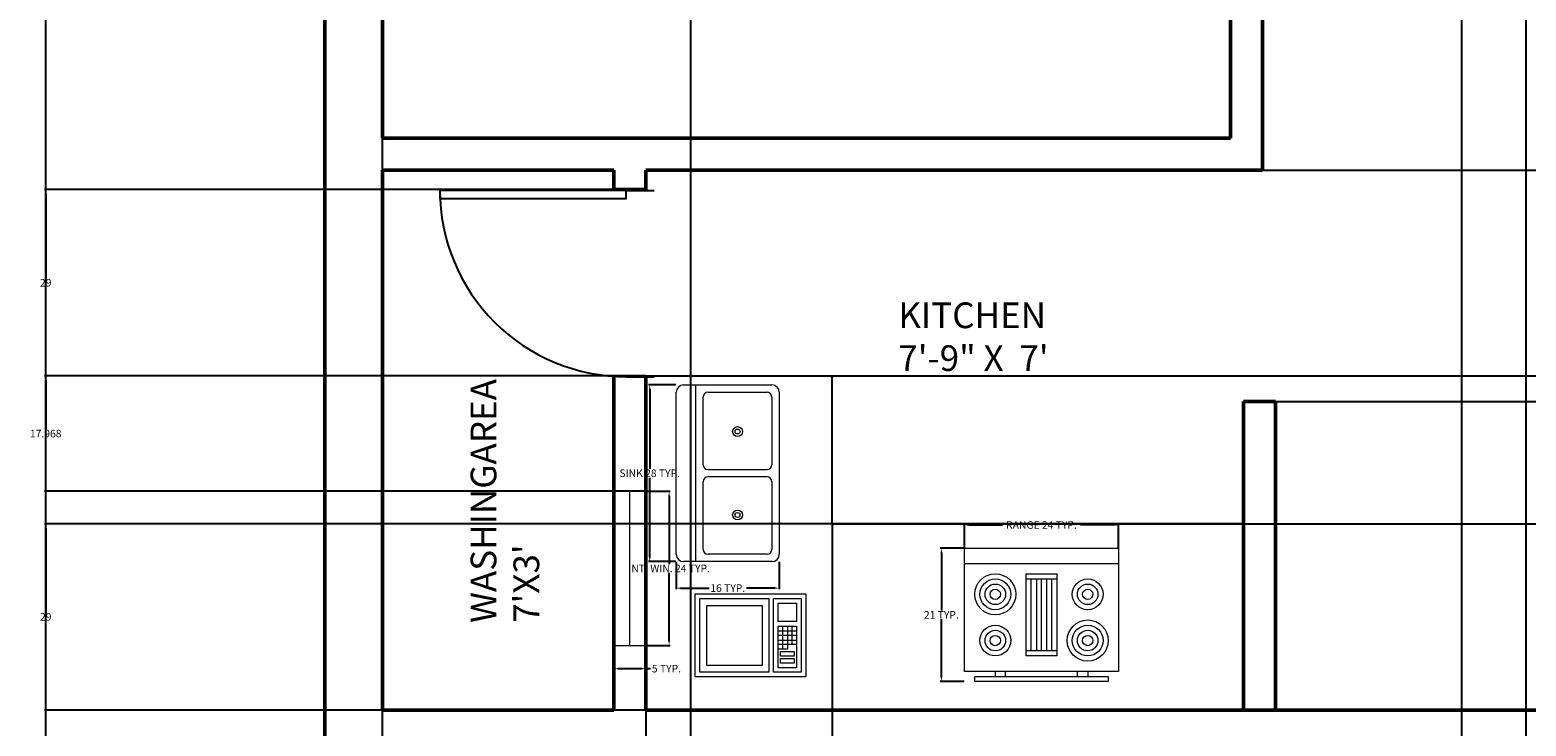
# Model space of a CAD drawing. Units: inches. Extents: x 3506 to 3958, y 1553 to 2506.
# Tile 13 of 16: x 3506 to 3739, y 2229 to 2337. Entities that reach past the tile are written whole.
import ezdxf

# ---------------------------------------------------------------- set-up
doc = ezdxf.new("R2010")
doc.units = ezdxf.units.IN
doc.header["$MEASUREMENT"] = 0
for name, color, linetype, lineweight in [('A-ANNO-DIMS', 2, 'Continuous', 18), ('A-AREA-IDEN', 7, 'Continuous', 18), ('A-FLOR-CASE', 7, 'Continuous', 25), ('A-WALL', 7, 'Continuous', 50), ('doors', 40, 'Continuous', 25), ('kitchen', 181, 'Continuous', 18), ('window', 30, 'Continuous', 20)]:
    doc.layers.add(name, color=color, linetype=linetype, lineweight=lineweight)
doc.layers.add('A-WALL-PATT', color=251, linetype='Continuous', lineweight=13, true_color=0x636466)
doc.styles.get("Standard").update_dxf_attribs({"font": 'arial.ttf'})
doc.dimstyles.get("Standard").update_dxf_attribs({"dimtxt": 1.18, "dimasz": 0.68, "dimexe": 0.18, "dimexo": 0.0625, "dimgap": 0.09, "dimtad": 0, "dimtih": 1, "dimtoh": 1, "dimdec": 1, "dimzin": 0, "dimdsep": 46, "dimlunit": 3, "dimtxsty": 'Standard', "dimcen": 0.09, "dimadec": 0, "dimazin": 0, "dimtfac": 1, "dimtdec": 1, "dimtofl": 0, "dimtmove": 0, "dimatfit": 3, "dimfxl": 1, "dimtolj": 1, "dimtzin": 0, "dimarcsym": 0})

# ---------------------------------------------------------------- blocks, each defined once
blk = doc.blocks.new('*U12')
for p, q in [((0, 0), (0, 6)), ((40, 0), (40, 6))]:
    blk.add_line(p, q)
blk.add_lwpolyline([(0, 0), (0, -40), (1.75, -40), (1.75, 0)], close=True)
blk.add_arc((0, 0), 40, 270, 0)
blk = doc.blocks.new('Microwave')
for p, q in [((18, 10), (22, 10)), ((19, 7), (19, 11)), ((20, 11), (20, 7)), ((21, 7), (21, 11)), ((22, 9), (18, 9)), ((18, 8), (22, 8)), ((22, 7), (18, 7)), ((19, 6), (19, 7)), ((20, 7), (20, 6)), ((20, 6), (18, 6))]:
    blk.add_line(p, q)
for points in [[(0, 0), (0, 18), (24, 18), (24, 0)], [(1, 1), (1, 17), (16, 17), (16, 1)], [(17, 1), (17, 17), (23, 17), (23, 1)], [(2.5, 2.5), (2.5, 15.5), (14.5, 15.5), (14.5, 2.5)], [(18, 12), (18, 16), (22, 16), (22, 12)], [(18, 2), (18, 11), (22, 11), (22, 2)], [(18.5, 4.5), (18.5, 5.5), (21.5, 5.5), (21.5, 4.5)], [(18.5, 3), (18.5, 4), (21.5, 4), (21.5, 3)]]:
    blk.add_lwpolyline(points, close=True)
blk = doc.blocks.new('Range-Oven - 30 in top')
for p, q in [((0, -3), (30, -3)), ((12, -6), (18, -6)), ((13, -20), (13, -6)), ((14, -6), (14, -20)), ((15, -20), (15, -6)), ((16, -6), (16, -20)), ((17, -20), (17, -6)), ((18, -20), (12, -20)), ((6, -24), (6, -25)), ((8, -25), (8, -24)), ((22, -25), (22, -24)), ((24, -24), (24, -25))]:
    blk.add_line(p, q)
for points in [[(0, -24), (0, 0), (30, 0), (30, -24)], [(12, -21), (12, -5), (18, -5), (18, -21)], [(2, -26), (2, -25), (28, -25), (28, -26)]]:
    blk.add_lwpolyline(points, close=True)
for centre, radius in [((6, -9), 4), ((6, -9), 3), ((6, -9), 2), ((6, -9), 1), ((24, -9), 3), ((24, -9), 2), ((24, -9), 1), ((24, -18), 4), ((6, -18), 3), ((6, -18), 2), ((6, -18), 1), ((24, -18), 3), ((24, -18), 2), ((24, -18), 1)]:
    blk.add_circle(centre, radius)
blk = doc.blocks.new('Sink-double - 36 in top')
for p, q in [((-18, -4), (18, -4)), ((-0.75, -18.5), (-0.75, -6.5)), ((0.75, -6.5), (0.75, -18.5))]:
    blk.add_line(p, q)
for points in [[(-16.5, 0), (16.5, 0)], [(-18, -19.5), (-18, -1.5)], [(18, -1.5), (18, -19.5)], [(-15.5, -5.5), (-1.75, -5.5)], [(1.75, -5.5), (15.5, -5.5)], [(-16.5, -18.5), (-16.5, -6.5)], [(16.5, -6.5), (16.5, -18.5)], [(16.5, -21), (-16.5, -21)], [(-1.75, -19.5), (-15.5, -19.5)], [(15.5, -19.5), (1.75, -19.5)]]:
    blk.add_lwpolyline(points)
for centre, radius in [((-8.5, -12.5), 1), ((-8.5, -12.5), 0.5), ((8.5, -12.5), 1), ((8.5, -12.5), 0.5)]:
    blk.add_circle(centre, radius)
for centre, radius, start, end in [((-16.5, -1.5), 1.5, 90, 180), ((16.5, -1.5), 1.5, 0, 90), ((-15.5, -6.5), 1, 90, 180), ((-1.75, -6.5), 1, 0, 90), ((1.75, -6.5), 1, 90, 180), ((15.5, -6.5), 1, 0, 90), ((-16.5, -19.5), 1.5, 180, 270), ((-15.5, -18.5), 1, 180, 270), ((-1.75, -18.5), 1, 270, 0), ((1.75, -18.5), 1, 180, 270), ((15.5, -18.5), 1, 270, 0), ((16.5, -19.5), 1.5, 270, 0)]:
    blk.add_arc(centre, radius, start, end)
blk = doc.blocks.new('WIN-24IN-5IN-PARTITION')
for p, q in [((5, 24), (0, 24)), ((0, 24), (0, 0)), ((2.5, 0), (2.5, 24)), ((5, 0), (5, 24)), ((0, 0), (5, 0)), ((0, 0), (2.5, 0))]:
    blk.add_line(p, q)
blk = doc.blocks.new('*D22')
at = {"layer": 'A-ANNO-DIMS', "color": 0, "lineweight": -2, "transparency": 16777216}
for p, q in [((3651.31, 2256.65), (3651.31, 2260.37)), ((3651.99, 2260.19), (3657.21, 2260.19)), ((3674.61, 2260.19), (3669.39, 2260.19)), ((3675.29, 2256.65), (3675.29, 2260.37))]:
    blk.add_line(p, q, dxfattribs=at)
at = {"layer": 'A-ANNO-DIMS', "color": 0, "transparency": 16777216}
for points in [[(3651.99, 2260.3), (3651.99, 2260.07), (3651.31, 2260.19)], [(3674.61, 2260.3), (3674.61, 2260.07), (3675.29, 2260.19)]]:
    blk.add_solid(points, dxfattribs=at)
at = {"layer": 'Defpoints', "color": 0, "transparency": 16777216}
for p in [(3675.29, 2260.19), (3651.31, 2256.59), (3675.29, 2256.59)]:
    blk.add_point(p, dxfattribs=at)
at = {"layer": 'A-ANNO-DIMS', "color": 0, "transparency": 16777216, "insert": (3663.3, 2260.19), "char_height": 1.18, "attachment_point": 5}
blk.add_mtext('\\A1;RANGE 24 TYP.', dxfattribs=at)
blk = doc.blocks.new('*D23')
at = {"layer": 'A-ANNO-DIMS', "color": 0, "lineweight": -2, "transparency": 16777216}
for p, q in [((3651.25, 2256.59), (3647.53, 2256.59)), ((3647.71, 2255.91), (3647.71, 2246.88)), ((3647.71, 2236.49), (3647.71, 2245.52)), ((3651.25, 2235.81), (3647.53, 2235.81))]:
    blk.add_line(p, q, dxfattribs=at)
at = {"layer": 'A-ANNO-DIMS', "color": 0, "transparency": 16777216}
for points in [[(3647.6, 2255.91), (3647.83, 2255.91), (3647.71, 2256.59)], [(3647.6, 2236.49), (3647.83, 2236.49), (3647.71, 2235.81)]]:
    blk.add_solid(points, dxfattribs=at)
at = {"layer": 'Defpoints', "color": 0, "transparency": 16777216}
for p in [(3647.71, 2256.59), (3651.31, 2256.59), (3651.31, 2235.81)]:
    blk.add_point(p, dxfattribs=at)
at = {"layer": 'A-ANNO-DIMS', "color": 0, "transparency": 16777216, "insert": (3647.71, 2246.2), "char_height": 1.18, "attachment_point": 5}
blk.add_mtext('\\A1;21 TYP.', dxfattribs=at)
blk = doc.blocks.new('*D24')
at = {"layer": 'A-ANNO-DIMS', "color": 0, "lineweight": -2, "transparency": 16777216}
for p, q in [((3606.38, 2281.99), (3602.13, 2281.99)), ((3602.31, 2281.31), (3602.31, 2268.94)), ((3602.31, 2255.17), (3602.31, 2267.54)), ((3606.38, 2254.49), (3602.13, 2254.49))]:
    blk.add_line(p, q, dxfattribs=at)
at = {"layer": 'A-ANNO-DIMS', "color": 0, "transparency": 16777216}
for points in [[(3602.2, 2281.31), (3602.43, 2281.31), (3602.31, 2281.99)], [(3602.2, 2255.17), (3602.43, 2255.17), (3602.31, 2254.49)]]:
    blk.add_solid(points, dxfattribs=at)
at = {"layer": 'Defpoints', "color": 0, "transparency": 16777216}
for p in [(3602.31, 2281.99), (3606.44, 2281.99), (3606.44, 2254.49)]:
    blk.add_point(p, dxfattribs=at)
at = {"layer": 'A-ANNO-DIMS', "color": 0, "transparency": 16777216, "insert": (3602.31, 2268.24), "char_height": 1.18, "attachment_point": 5}
blk.add_mtext('\\A1;SINK 28 TYP.', dxfattribs=at)
blk = doc.blocks.new('*D25')
at = {"layer": 'A-ANNO-DIMS', "color": 0, "lineweight": -2, "transparency": 16777216}
for p, q in [((3606.44, 2254.43), (3606.44, 2250.18)), ((3622.48, 2254.43), (3622.48, 2250.18)), ((3607.12, 2250.36), (3611.55, 2250.36)), ((3621.8, 2250.36), (3617.36, 2250.36))]:
    blk.add_line(p, q, dxfattribs=at)
at = {"layer": 'A-ANNO-DIMS', "color": 0, "transparency": 16777216}
for points in [[(3607.12, 2250.48), (3607.12, 2250.25), (3606.44, 2250.36)], [(3621.8, 2250.48), (3621.8, 2250.25), (3622.48, 2250.36)]]:
    blk.add_solid(points, dxfattribs=at)
at = {"layer": 'Defpoints', "color": 0, "transparency": 16777216}
for p in [(3606.44, 2254.49), (3622.48, 2254.49), (3606.44, 2250.36)]:
    blk.add_point(p, dxfattribs=at)
at = {"layer": 'A-ANNO-DIMS', "color": 0, "transparency": 16777216, "insert": (3614.46, 2250.36), "char_height": 1.18, "attachment_point": 5}
blk.add_mtext('\\A1;16 TYP.', dxfattribs=at)
blk = doc.blocks.new('*D34')
at = {"layer": 'A-ANNO-DIMS', "color": 0, "lineweight": -2, "transparency": 16777216}
for p, q in [((3601.79, 2265.43), (3605.51, 2265.43)), ((3605.33, 2264.75), (3605.33, 2254.11)), ((3605.33, 2242.11), (3605.33, 2252.74)), ((3601.79, 2241.43), (3605.51, 2241.43))]:
    blk.add_line(p, q, dxfattribs=at)
at = {"layer": 'A-ANNO-DIMS', "color": 0, "transparency": 16777216}
for points in [[(3605.22, 2264.75), (3605.44, 2264.75), (3605.33, 2265.43)], [(3605.22, 2242.11), (3605.44, 2242.11), (3605.33, 2241.43)]]:
    blk.add_solid(points, dxfattribs=at)
at = {"layer": 'Defpoints', "color": 0, "transparency": 16777216}
for p in [(3601.73, 2265.43), (3605.33, 2265.43), (3601.73, 2241.43)]:
    blk.add_point(p, dxfattribs=at)
at = {"layer": 'A-ANNO-DIMS', "color": 0, "transparency": 16777216, "insert": (3605.33, 2253.43), "char_height": 1.18, "attachment_point": 5}
blk.add_mtext('\\A1;INT. WIN. 24 TYP.', dxfattribs=at)
blk = doc.blocks.new('*D35')
at = {"layer": 'A-ANNO-DIMS', "color": 0, "lineweight": -2, "transparency": 16777216}
for p, q in [((3596.73, 2241.36), (3596.73, 2237.65)), ((3601.73, 2241.36), (3601.73, 2237.65)), ((3597.41, 2237.83), (3601.05, 2237.83)), ((3601.73, 2237.83), (3602.41, 2237.83))]:
    blk.add_line(p, q, dxfattribs=at)
at = {"layer": 'A-ANNO-DIMS', "color": 0, "transparency": 16777216}
for points in [[(3597.41, 2237.94), (3597.41, 2237.71), (3596.73, 2237.83)], [(3601.05, 2237.94), (3601.05, 2237.71), (3601.73, 2237.83)]]:
    blk.add_solid(points, dxfattribs=at)
at = {"layer": 'Defpoints', "color": 0, "transparency": 16777216}
for p in [(3596.73, 2241.43), (3601.73, 2241.43), (3601.73, 2237.83)]:
    blk.add_point(p, dxfattribs=at)
at = {"layer": 'A-ANNO-DIMS', "color": 0, "transparency": 16777216, "insert": (3604.91, 2237.83), "char_height": 1.18, "attachment_point": 5}
blk.add_mtext('\\A1;5 TYP.', dxfattribs=at)
blk = doc.blocks.new('*D44')
at = {"layer": 'A-ANNO-DIMS', "color": 0, "lineweight": -2, "transparency": 16777216}
for p, q in [((3911.67, 2461.39), (3508.1, 2461.39)), ((3508.28, 2460.71), (3508.28, 2344.59)), ((3508.28, 2227.07), (3508.28, 2343.2)), ((3560.67, 2226.39), (3508.1, 2226.39))]:
    blk.add_line(p, q, dxfattribs=at)
at = {"layer": 'A-ANNO-DIMS', "color": 0, "transparency": 16777216}
for points in [[(3508.17, 2460.71), (3508.39, 2460.71), (3508.28, 2461.39)], [(3508.17, 2227.07), (3508.39, 2227.07), (3508.28, 2226.39)]]:
    blk.add_solid(points, dxfattribs=at)
at = {"layer": 'Defpoints', "color": 0, "transparency": 16777216}
for p in [(3508.28, 2461.39), (3911.73, 2461.39), (3560.73, 2226.39)]:
    blk.add_point(p, dxfattribs=at)
at = {"layer": 'A-ANNO-DIMS', "color": 0, "transparency": 16777216, "insert": (3508.28, 2343.89), "char_height": 1.18, "attachment_point": 5}
blk.add_mtext('\\A1;235', dxfattribs=at)
blk = doc.blocks.new('*D50')
at = {"layer": 'A-ANNO-DIMS', "color": 0, "lineweight": -2, "transparency": 16777216}
for p, q in [((3608.73, 1606.46), (3608.73, 2505.02)), ((3609.41, 2504.84), (3672.39, 2504.84)), ((3738.05, 2504.84), (3675.07, 2504.84)), ((3738.73, 1606.46), (3738.73, 2505.02))]:
    blk.add_line(p, q, dxfattribs=at)
at = {"layer": 'A-ANNO-DIMS', "color": 0, "transparency": 16777216}
for points in [[(3609.41, 2504.96), (3609.41, 2504.73), (3608.73, 2504.84)], [(3738.05, 2504.96), (3738.05, 2504.73), (3738.73, 2504.84)]]:
    blk.add_solid(points, dxfattribs=at)
at = {"layer": 'Defpoints', "color": 0, "transparency": 16777216}
for p in [(3738.73, 2504.84), (3608.73, 1606.39), (3738.73, 1606.39)]:
    blk.add_point(p, dxfattribs=at)
at = {"layer": 'A-ANNO-DIMS', "color": 0, "transparency": 16777216, "insert": (3673.73, 2504.84), "char_height": 1.18, "attachment_point": 5}
blk.add_mtext('\\A1;130', dxfattribs=at)
blk = doc.blocks.new('*D52')
at = {"layer": 'A-ANNO-DIMS', "color": 0, "lineweight": -2, "transparency": 16777216}
for p, q in [((3560.73, 1606.46), (3560.73, 2505.02)), ((3561.41, 2504.84), (3583.77, 2504.84)), ((3608.05, 2504.84), (3585.69, 2504.84)), ((3608.73, 1606.46), (3608.73, 2505.02))]:
    blk.add_line(p, q, dxfattribs=at)
at = {"layer": 'A-ANNO-DIMS', "color": 0, "transparency": 16777216}
for points in [[(3561.41, 2504.96), (3561.41, 2504.73), (3560.73, 2504.84)], [(3608.05, 2504.96), (3608.05, 2504.73), (3608.73, 2504.84)]]:
    blk.add_solid(points, dxfattribs=at)
at = {"layer": 'Defpoints', "color": 0, "transparency": 16777216}
for p in [(3608.73, 2504.84), (3560.73, 1606.39), (3608.73, 1606.39)]:
    blk.add_point(p, dxfattribs=at)
at = {"layer": 'A-ANNO-DIMS', "color": 0, "transparency": 16777216, "insert": (3584.73, 2504.84), "char_height": 1.18, "attachment_point": 5}
blk.add_mtext('\\A1;48', dxfattribs=at)
blk = doc.blocks.new('*D58')
at = {"layer": 'A-ANNO-DIMS', "color": 0, "lineweight": -2, "transparency": 16777216}
for p, q in [((3596.67, 2312.39), (3508.1, 2312.39)), ((3508.28, 2311.71), (3508.28, 2298.59)), ((3508.28, 2284.07), (3508.28, 2297.2)), ((3596.67, 2283.39), (3508.1, 2283.39))]:
    blk.add_line(p, q, dxfattribs=at)
at = {"layer": 'A-ANNO-DIMS', "color": 0, "transparency": 16777216}
for points in [[(3508.17, 2311.71), (3508.39, 2311.71), (3508.28, 2312.39)], [(3508.17, 2284.07), (3508.39, 2284.07), (3508.28, 2283.39)]]:
    blk.add_solid(points, dxfattribs=at)
at = {"layer": 'Defpoints', "color": 0, "transparency": 16777216}
for p in [(3596.73, 2312.39), (3508.28, 2283.39), (3596.73, 2283.39)]:
    blk.add_point(p, dxfattribs=at)
at = {"layer": 'A-ANNO-DIMS', "color": 0, "transparency": 16777216, "insert": (3508.28, 2297.89), "char_height": 1.18, "attachment_point": 5}
blk.add_mtext('\\A1;29', dxfattribs=at)
blk = doc.blocks.new('*D59')
at = {"layer": 'A-ANNO-DIMS', "color": 0, "lineweight": -2, "transparency": 16777216}
for p, q in [((3728.73, 1689.46), (3728.73, 2505.02)), ((3729.41, 2504.84), (3732.85, 2504.84)), ((3738.05, 2504.84), (3734.61, 2504.84)), ((3738.73, 1689.46), (3738.73, 2505.02))]:
    blk.add_line(p, q, dxfattribs=at)
at = {"layer": 'A-ANNO-DIMS', "color": 0, "transparency": 16777216}
for points in [[(3729.41, 2504.96), (3729.41, 2504.73), (3728.73, 2504.84)], [(3738.05, 2504.96), (3738.05, 2504.73), (3738.73, 2504.84)]]:
    blk.add_solid(points, dxfattribs=at)
at = {"layer": 'Defpoints', "color": 0, "transparency": 16777216}
for p in [(3738.73, 2504.84), (3728.73, 1689.39), (3738.73, 1689.39)]:
    blk.add_point(p, dxfattribs=at)
at = {"layer": 'A-ANNO-DIMS', "color": 0, "transparency": 16777216, "insert": (3733.73, 2504.84), "char_height": 1.18, "attachment_point": 5}
blk.add_mtext('\\A1;10', dxfattribs=at)
blk = doc.blocks.new('*D67')
at = {"layer": 'A-ANNO-DIMS', "color": 0, "lineweight": -2, "transparency": 16777216}
for p, q in [((3697.79, 2315.39), (3955.36, 2315.39)), ((3955.18, 2314.71), (3955.18, 2298.09)), ((3955.18, 2280.07), (3955.18, 2296.7)), ((3699.79, 2279.39), (3955.36, 2279.39))]:
    blk.add_line(p, q, dxfattribs=at)
at = {"layer": 'A-ANNO-DIMS', "color": 0, "transparency": 16777216}
for points in [[(3955.07, 2314.71), (3955.29, 2314.71), (3955.18, 2315.39)], [(3955.07, 2280.07), (3955.29, 2280.07), (3955.18, 2279.39)]]:
    blk.add_solid(points, dxfattribs=at)
at = {"layer": 'Defpoints', "color": 0, "transparency": 16777216}
for p in [(3697.73, 2315.39), (3699.73, 2279.39), (3955.18, 2279.39)]:
    blk.add_point(p, dxfattribs=at)
at = {"layer": 'A-ANNO-DIMS', "color": 0, "transparency": 16777216, "insert": (3955.18, 2297.39), "char_height": 1.18, "attachment_point": 5}
blk.add_mtext('\\A1;36', dxfattribs=at)
blk = doc.blocks.new('*D68')
at = {"layer": 'A-ANNO-DIMS', "color": 0, "lineweight": -2, "transparency": 16777216}
for p, q in [((3630.73, 2260.33), (3630.73, 1553.76)), ((3601.73, 2231.33), (3601.73, 1553.76)), ((3602.41, 1553.94), (3615.28, 1553.94)), ((3630.05, 1553.94), (3617.18, 1553.94))]:
    blk.add_line(p, q, dxfattribs=at)
at = {"layer": 'A-ANNO-DIMS', "color": 0, "transparency": 16777216}
for points in [[(3602.41, 1554.06), (3602.41, 1553.83), (3601.73, 1553.94)], [(3630.05, 1554.06), (3630.05, 1553.83), (3630.73, 1553.94)]]:
    blk.add_solid(points, dxfattribs=at)
at = {"layer": 'Defpoints', "color": 0, "transparency": 16777216}
for p in [(3630.73, 2260.39), (3601.73, 2231.39), (3630.73, 1553.94)]:
    blk.add_point(p, dxfattribs=at)
at = {"layer": 'A-ANNO-DIMS', "color": 0, "transparency": 16777216, "insert": (3616.23, 1553.94), "char_height": 1.18, "attachment_point": 5}
blk.add_mtext('\\A1;29', dxfattribs=at)
blk = doc.blocks.new('*D69')
at = {"layer": 'A-ANNO-DIMS', "color": 0, "lineweight": -2, "transparency": 16777216}
for p, q in [((3630.79, 2283.39), (3955.36, 2283.39)), ((3955.18, 2282.71), (3955.18, 2272.59)), ((3955.18, 2261.07), (3955.18, 2271.2)), ((3630.79, 2260.39), (3955.36, 2260.39))]:
    blk.add_line(p, q, dxfattribs=at)
at = {"layer": 'A-ANNO-DIMS', "color": 0, "transparency": 16777216}
for points in [[(3955.07, 2282.71), (3955.29, 2282.71), (3955.18, 2283.39)], [(3955.07, 2261.07), (3955.29, 2261.07), (3955.18, 2260.39)]]:
    blk.add_solid(points, dxfattribs=at)
at = {"layer": 'Defpoints', "color": 0, "transparency": 16777216}
for p in [(3630.73, 2283.39), (3630.73, 2260.39), (3955.18, 2260.39)]:
    blk.add_point(p, dxfattribs=at)
at = {"layer": 'A-ANNO-DIMS', "color": 0, "transparency": 16777216, "insert": (3955.18, 2271.89), "char_height": 1.18, "attachment_point": 5}
blk.add_mtext('\\A1;23', dxfattribs=at)
blk = doc.blocks.new('*D70')
at = {"layer": 'A-ANNO-DIMS', "color": 0, "lineweight": -2, "transparency": 16777216}
for p, q in [((3694.67, 2260.39), (3508.1, 2260.39)), ((3508.28, 2259.71), (3508.28, 2246.59)), ((3508.28, 2232.07), (3508.28, 2245.2)), ((3694.67, 2231.39), (3508.1, 2231.39))]:
    blk.add_line(p, q, dxfattribs=at)
at = {"layer": 'A-ANNO-DIMS', "color": 0, "transparency": 16777216}
for points in [[(3508.17, 2259.71), (3508.39, 2259.71), (3508.28, 2260.39)], [(3508.17, 2232.07), (3508.39, 2232.07), (3508.28, 2231.39)]]:
    blk.add_solid(points, dxfattribs=at)
at = {"layer": 'Defpoints', "color": 0, "transparency": 16777216}
for p in [(3694.73, 2260.39), (3508.28, 2231.39), (3694.73, 2231.39)]:
    blk.add_point(p, dxfattribs=at)
at = {"layer": 'A-ANNO-DIMS', "color": 0, "transparency": 16777216, "insert": (3508.28, 2245.89), "char_height": 1.18, "attachment_point": 5}
blk.add_mtext('\\A1;29', dxfattribs=at)
blk = doc.blocks.new('*D71')
at = {"layer": 'A-ANNO-DIMS', "color": 0, "lineweight": -2, "transparency": 16777216}
for p, q in [((3601.67, 2283.39), (3508.1, 2283.39)), ((3508.28, 2282.71), (3508.28, 2275.1)), ((3508.28, 2266.11), (3508.28, 2273.72)), ((3601.67, 2265.43), (3508.1, 2265.43))]:
    blk.add_line(p, q, dxfattribs=at)
at = {"layer": 'A-ANNO-DIMS', "color": 0, "transparency": 16777216}
for points in [[(3508.17, 2282.71), (3508.39, 2282.71), (3508.28, 2283.39)], [(3508.17, 2266.11), (3508.39, 2266.11), (3508.28, 2265.43)]]:
    blk.add_solid(points, dxfattribs=at)
at = {"layer": 'Defpoints', "color": 0, "transparency": 16777216}
for p in [(3508.28, 2283.39), (3601.73, 2283.39), (3601.73, 2265.43)]:
    blk.add_point(p, dxfattribs=at)
at = {"layer": 'A-ANNO-DIMS', "color": 0, "transparency": 16777216, "insert": (3508.28, 2274.41), "char_height": 1.18, "attachment_point": 5}
blk.add_mtext('\\A1;17.968', dxfattribs=at)

msp = doc.modelspace()

# ---------------------------------------------------------------- hatches: boundary and pattern name
at = {"layer": 'A-WALL-PATT'}
h = msp.add_hatch(dxfattribs=at)
h.set_pattern_fill('ANSI31', color=256)
h.paths.add_polyline_path([(3911.7302, 2461.3942), (3551.7302, 2461.3942), (3551.7302, 2152.516), (3560.7302, 2152.516), (3560.7302, 2116.516), (3551.7302, 2116.516), (3551.7302, 1920.5711), (3556.2302, 1920.5711), (3560.7302, 1920.5711), (3560.7302, 2000.3942), (3692.7302, 2000.3942), (3692.7302, 1997.3942), (3697.7302, 1997.3942), (3697.7302, 2000.3942), (3771.7302, 2000.3942), (3771.7302, 1997.3942), (3776.7302, 1997.3942), (3776.7302, 1997.7206), (3778.5802, 1997.7206), (3807.5802, 1997.7206), (3807.5802, 1996.4519), (3778.5802, 1996.4519), (3778.5802, 1997.7206), (3776.7302, 1997.7206), (3776.7302, 1997.3942), (3771.7302, 1997.3942), (3771.7302, 2000.3942), (3697.7302, 2000.3942), (3697.7302, 1997.3942), (3692.7302, 1997.3942), (3689.8302, 1997.3942), (3689.8302, 1995.8192), (3653.8302, 1995.8192), (3653.8302, 1997.3942), (3689.8302, 1997.3942), (3692.7302, 1997.3942), (3692.7302, 2000.3942), (3560.7302, 2000.3942), (3560.7302, 1920.5711), (3551.7302, 1920.5711), (3551.7302, 1884.5711), (3551.7302, 1597.3942), (3911.7302, 1597.3942)], flags=17)
h.paths.add_polyline_path([(3596.7302, 2005.3942), (3596.7302, 2057.3035, -0.38730371), (3569.1778, 2085), (3569.15, 2085), (3569.15, 2086.2688), (3598.15, 2086.2688), (3598.15, 2085), (3569.1778, 2085, 0.38730371), (3596.7302, 2057.3035), (3596.7302, 2057.3942), (3601.7302, 2057.3942), (3601.7302, 2055.3942), (3630.7302, 2055.3942), (3630.7302, 2034.3942), (3694.7302, 2034.3942), (3694.7302, 2053.3942), (3699.7302, 2053.3942), (3699.7302, 2005.3942), (3860.7302, 2005.3942), (3860.7302, 2173.3942), (3771.7302, 2173.3942), (3771.7302, 2194.3942), (3776.7302, 2194.3942), (3776.7302, 2178.3942), (3860.7302, 2178.3942), (3860.7302, 2231.3942), (3601.7302, 2231.3942), (3601.7302, 2241.426), (3596.7302, 2241.426), (3596.7302, 2231.3942), (3560.7302, 2231.3942), (3560.7302, 2315.3942), (3596.7302, 2315.3942), (3596.7302, 2312.3942), (3601.7302, 2312.3942), (3601.7302, 2315.3942), (3697.7302, 2315.3942), (3697.7302, 2413.3942), (3692.7302, 2413.3942), (3692.7302, 2320.3942), (3560.7302, 2320.3942), (3560.7302, 2452.3942), (3692.7302, 2452.3942), (3692.7302, 2449.3942), (3697.7302, 2449.3942), (3697.7302, 2452.3942), (3771.7302, 2452.3942), (3771.7302, 2449.3942), (3776.7302, 2449.3942), (3776.7302, 2452.3942), (3860.7302, 2452.3942), (3860.7302, 2437.2075), (3865.2302, 2437.2075), (3865.2302, 2413.2075), (3860.7302, 2413.2075), (3860.7302, 2367.6976), (3865.2302, 2367.6976), (3869.7302, 2367.6976), (3869.7302, 2319.6976), (3860.7302, 2319.6976), (3860.7302, 2211.6248), (3869.7302, 2211.6248), (3869.7302, 2187.6248), (3860.7302, 2187.6248), (3860.7302, 2138.4346), (3865.2302, 2138.4346), (3869.7302, 2138.4346), (3869.7302, 2090.4346), (3860.7302, 2090.4346), (3860.7302, 1985.8449), (3869.7302, 1985.8449), (3869.7302, 1961.8449), (3860.7302, 1961.8449), (3860.7302, 1897.0756), (3865.2302, 1897.0756), (3869.7302, 1897.0756), (3869.7302, 1849.0756), (3860.7302, 1849.0756), (3860.7302, 1847.8112), (3860.7302, 1779.3942), (3596.7302, 1779.3942), (3596.7302, 1831.3942), (3601.7302, 1831.3942), (3601.7302, 1828.3942), (3630.7302, 1828.3942), (3630.7302, 1808.3942), (3691.7302, 1808.3942), (3691.7302, 1815.3942), (3696.7302, 1815.3942), (3696.7302, 1779.3942), (3860.7302, 1779.3942), (3860.7302, 1947.3942), (3771.7302, 1947.3942), (3771.7302, 1968.3942), (3776.7302, 1968.3942), (3776.7302, 1952.3942), (3860.7302, 1952.3942), (3860.7302, 2005.3942)], flags=0)
h.paths.add_polyline_path([(3596.7302, 2038.8546), (3601.7302, 2038.8546), (3601.7302, 2014.8546), (3596.7302, 2014.8546)], flags=0)
h.paths.add_polyline_path([(3564.1688, 2107), (3564.1688, 2167), (3644.1688, 2167), (3644.1688, 2107)], flags=0)
h.paths.add_polyline_path([(3607.0972, 2052.0208), (3620.8472, 2052.0208, -0.41421356), (3621.9931, 2050.875), (3621.9931, 2025.6667, -0.41421356), (3620.8472, 2024.5208), (3607.0972, 2024.5208, -0.41421356), (3605.9514, 2025.6667), (3605.9514, 2050.875, -0.41421356)], flags=0)
h.paths.add_polyline_path([(3578.5688, 2115), (3565.3688, 2115), (3565.3688, 2135.8), (3578.5688, 2135.8), (3578.5688, 2138.2), (3565.3688, 2138.2), (3565.3688, 2159), (3580.5688, 2159), (3580.5688, 2153.8), (3593.7688, 2167), (3593.7688, 2151.8), (3578.5688, 2151.8)], flags=0)
h.paths.add_polyline_path([(3610.9167, 2050.875), (3620.0833, 2050.875, -0.41421356), (3620.8472, 2050.1111), (3620.8472, 2039.6076, -0.41421356), (3620.0833, 2038.8438), (3610.9167, 2038.8438, -0.41421356), (3610.1528, 2039.6076), (3610.1528, 2050.1111, -0.41421356)], flags=0)
h.paths.add_polyline_path([(3610.9167, 2037.6979), (3620.0833, 2037.6979, -0.41421356), (3620.8472, 2036.934), (3620.8472, 2026.4306, -0.41421356), (3620.0833, 2025.6667), (3610.9167, 2025.6667, -0.41421356), (3610.1528, 2026.4306), (3610.1528, 2036.934, -0.41421356)], flags=0)
h.paths.add_polyline_path([(3616.2639, 2044.7639, -1), (3614.7361, 2044.7639, -1)], flags=0)
h.paths.add_polyline_path([(3615.8819, 2044.7639, -1), (3615.1181, 2044.7639, -1)], flags=0)
h.paths.add_polyline_path([(3616.2639, 2031.7778, -1), (3614.7361, 2031.7778, -1)], flags=0)
h.paths.add_polyline_path([(3615.8819, 2031.7778, -1), (3615.1181, 2031.7778, -1)], flags=0)
h.paths.add_polyline_path([(3609.7539, 2021.7868), (3626.9586, 2021.7868), (3626.9586, 2008.8833), (3609.7539, 2008.8833)], flags=0)
h.paths.add_polyline_path([(3610.4708, 2021.07), (3621.2237, 2021.07), (3621.2237, 2009.6002), (3610.4708, 2009.6002)], flags=0)
h.paths.add_polyline_path([(3611.5461, 2019.9947), (3620.1484, 2019.9947), (3620.1484, 2010.6755), (3611.5461, 2010.6755)], flags=0)
h.paths.add_polyline_path([(3621.9405, 2021.07), (3626.2417, 2021.07), (3626.2417, 2009.6002), (3621.9405, 2009.6002)], flags=0)
h.paths.add_polyline_path([(3622.6574, 2020.3531), (3625.5248, 2020.3531), (3625.5248, 2017.4857), (3622.6574, 2017.4857)], flags=0)
h.paths.add_polyline_path([(3622.6574, 2016.7688), (3625.5248, 2016.7688), (3625.5248, 2010.317), (3622.6574, 2010.317)], flags=0)
h.paths.add_polyline_path([(3624.808, 2016.0519), (3624.808, 2013.9013), (3624.0911, 2013.9013), (3624.0911, 2013.1845), (3623.3743, 2013.1845), (3623.3743, 2013.9013), (3623.3743, 2016.0519)], flags=0)
h.paths.add_polyline_path([(3623.0158, 2012.8261), (3625.1664, 2012.8261), (3625.1664, 2012.1092), (3623.0158, 2012.1092)], flags=0)
h.paths.add_polyline_path([(3623.0158, 2011.7508), (3625.1664, 2011.7508), (3625.1664, 2011.0339), (3623.0158, 2011.0339)], flags=0)
h.paths.add_polyline_path([(3650.0591, 2031.8202), (3674.0368, 2031.8202), (3674.0368, 2012.638), (3669.2413, 2012.638), (3669.2413, 2011.8388), (3672.4383, 2011.8388), (3672.4383, 2011.0395), (3651.6576, 2011.0395), (3651.6576, 2011.8388), (3654.8546, 2011.8388), (3654.8546, 2012.638), (3650.0591, 2012.638)], flags=0)
h.paths.add_polyline_path([(3658.0517, 2024.6269, -1), (3651.6576, 2024.6269, -1)], flags=0)
h.paths.add_polyline_path([(3657.2524, 2024.6269, -1), (3652.4569, 2024.6269, -1)], flags=0)
h.paths.add_polyline_path([(3656.4532, 2024.6269, -1), (3653.2561, 2024.6269, -1)], flags=0)
h.paths.add_polyline_path([(3655.6539, 2024.6269, -1), (3654.0554, 2024.6269, -1)], flags=0)
h.paths.add_polyline_path([(3657.2524, 2017.4336, -1), (3652.4569, 2017.4336, -1)], flags=0)
h.paths.add_polyline_path([(3656.4532, 2017.4336, -1), (3653.2561, 2017.4336, -1)], flags=0)
h.paths.add_polyline_path([(3655.6539, 2017.4336, -1), (3654.0554, 2017.4336, -1)], flags=0)
h.paths.add_polyline_path([(3659.6502, 2027.8239), (3664.4457, 2027.8239), (3664.4457, 2015.0358), (3659.6502, 2015.0358)], flags=0)
h.paths.add_polyline_path([(3663.6465, 2027.0247), (3663.6465, 2015.8351), (3660.4494, 2015.8351), (3660.4494, 2027.0247)], flags=0)
h.paths.add_polyline_path([(3562.6688, 1945.5), (3642.6688, 1945.5), (3642.6688, 1885.5), (3562.6688, 1885.5)], flags=0)
h.paths.add_polyline_path([(3671.6391, 2024.6269, -1), (3666.8435, 2024.6269, -1)], flags=0)
h.paths.add_polyline_path([(3670.8398, 2024.6269, -1), (3667.6428, 2024.6269, -1)], flags=0)
h.paths.add_polyline_path([(3672.4383, 2017.4336, -1), (3666.0443, 2017.4336, -1)], flags=0)
h.paths.add_polyline_path([(3670.0405, 2024.6269, -1), (3668.442, 2024.6269, -1)], flags=0)
h.paths.add_polyline_path([(3671.6391, 2017.4336, -1), (3666.8435, 2017.4336, -1)], flags=0)
h.paths.add_polyline_path([(3670.8398, 2017.4336, -1), (3667.6428, 2017.4336, -1)], flags=0)
h.paths.add_polyline_path([(3592.2688, 1945.5), (3592.2688, 1930.3), (3577.0688, 1930.3), (3577.0688, 1893.5), (3563.8688, 1893.5), (3563.8688, 1914.3), (3577.0688, 1914.3), (3577.0688, 1916.7), (3563.8688, 1916.7), (3563.8688, 1937.5), (3579.0688, 1937.5), (3579.0688, 1932.3)], flags=0)
h.paths.add_polyline_path([(3670.0405, 2017.4336, -1), (3668.442, 2017.4336, -1)], flags=0)
h.paths.add_polyline_path([(3596.7302, 2283.3942), (3601.7302, 2283.3942), (3601.7302, 2265.426), (3599.2302, 2265.426), (3599.2302, 2241.426), (3596.7302, 2241.426), (3596.7302, 2265.426)], flags=0)
h.paths.add_polyline_path([(3596.7302, 1810.7006), (3601.7302, 1810.7006), (3601.7302, 1786.7006), (3596.7302, 1786.7006)], flags=0)
h.paths.add_polyline_path([(3560.7302, 1770.3942), (3738.7302, 1770.3942), (3738.7302, 1746.3942), (3738.7302, 1722.3942), (3748.7302, 1722.3942), (3748.7302, 1674.3942), (3560.7302, 1674.3942)], flags=0)
h.paths.add_polyline_path([(3728.7302, 1746.3942), (3728.7302, 1756.0642), (3738.7302, 1746.3942), (3728.7302, 1738.1582), (3728.7302, 1698.3942), (3591.2519, 1698.3942), (3591.2519, 1746.3942)], flags=0)
h.paths.add_polyline_path([(3771.7302, 2399.3942), (3771.7302, 2420.3942), (3776.7302, 2420.3942), (3776.7302, 2404.3942), (3776.7302, 2399.3942)], flags=0)
h.paths.add_polyline_path([(3911.7302, 2461.3942), (3551.7302, 2461.3942), (3551.7302, 2152.516), (3560.7302, 2152.516), (3560.7302, 2116.516), (3551.7302, 2116.516), (3551.7302, 1920.5711), (3560.7302, 1920.5711), (3560.7302, 2000.3942), (3692.7302, 2000.3942), (3692.7302, 1997.3942), (3697.7302, 1997.3942), (3697.7302, 2000.3942), (3771.7302, 2000.3942), (3771.7302, 1997.3942), (3776.7302, 1997.3942), (3776.7302, 1997.7206), (3778.5802, 1997.7206), (3807.5802, 1997.7206), (3807.5802, 1996.4519), (3778.5802, 1996.4519), (3778.5802, 1997.7206), (3776.7302, 1997.7206), (3776.7302, 1997.3942), (3771.7302, 1997.3942), (3771.7302, 2000.3942), (3697.7302, 2000.3942), (3697.7302, 1997.3942), (3692.7302, 1997.3942), (3689.8302, 1997.3942), (3689.8302, 1995.8192), (3653.8302, 1995.8192), (3653.8302, 1997.3942), (3689.8302, 1997.3942), (3692.7302, 1997.3942), (3692.7302, 2000.3942), (3560.7302, 2000.3942), (3560.7302, 1920.5711), (3551.7302, 1920.5711), (3551.7302, 1597.3942), (3911.7302, 1597.3942)], flags=17)

# ---------------------------------------------------------------- linework, layer by layer
at = {"layer": 'A-FLOR-CASE'}
for p, q in [((3596.7302, 2283.3942), (3630.7302, 2283.3942)), ((3630.7302, 2260.3942), (3630.7302, 2283.3942)), ((3630.7302, 2260.3942), (3694.7302, 2260.3942))]:
    msp.add_line(p, q, dxfattribs=at)
at = {"layer": 'A-WALL'}
for p, q in [((3560.7302, 2320.3942), (3560.7302, 2452.3942)), ((3692.7302, 2320.3942), (3692.7302, 2413.3942)), ((3692.7302, 2320.3942), (3692.7302, 2413.3942)), ((3697.7302, 2320.3942), (3697.7302, 2413.3942)), ((3697.7302, 2315.3942), (3697.7302, 2413.3942)), ((3560.7302, 2320.3942), (3692.7302, 2320.3942)), ((3560.7302, 2315.3942), (3596.7302, 2315.3942)), ((3560.7302, 2231.3942), (3560.7302, 2315.3942)), ((3596.7302, 2315.3942), (3596.7302, 2312.3942)), ((3596.7302, 2312.3942), (3596.7302, 2315.3942)), ((3596.7302, 2312.3942), (3596.7302, 2315.3942)), ((3601.7302, 2315.3942), (3697.7302, 2315.3942)), ((3601.7302, 2312.3942), (3601.7302, 2315.3942)), ((3601.7302, 2312.3942), (3601.7302, 2315.3942)), ((3596.7302, 2312.3942), (3601.7302, 2312.3942)), ((3596.7302, 2231.3942), (3596.7302, 2283.3942)), ((3596.7302, 2231.3942), (3596.7302, 2283.3942)), ((3601.7302, 2231.3942), (3601.7302, 2283.3942)), ((3601.7302, 2231.3942), (3601.7302, 2283.3942)), ((3694.7302, 2231.3942), (3694.7302, 2279.3942)), ((3694.7302, 2279.3942), (3699.7302, 2279.3942)), ((3699.7302, 2231.3942), (3699.7302, 2279.3942)), ((3560.7302, 2231.3942), (3596.7302, 2231.3942)), ((3601.7302, 2231.3942), (3860.7302, 2231.3942))]:
    msp.add_line(p, q, dxfattribs=at)
msp.add_lwpolyline([(3551.7302, 2461.3942), (3911.7302, 2461.3942), (3911.7302, 1597.3942), (3551.7302, 1597.3942)], close=True, dxfattribs=at)

# ---------------------------------------------------------------- block references
at = {"layer": 'doors', "xscale": 0.725, "yscale": 0.725, "zscale": 0.725, "rotation": 270}
msp.add_blockref('*U12', (3598.65, 2312.2688), dxfattribs=at)
at = {"layer": 'kitchen', "xscale": 0.763888888888889, "yscale": 0.763888888888889, "zscale": 0.763888888888889, "rotation": 90}
msp.add_blockref('Sink-double - 36 in top', (3606.4375, 2268.2378), dxfattribs=at)
at = {"layer": 'kitchen'}
for name, p, xscale, yscale, zscale in [('Range-Oven - 30 in top', (3651.3104, 2256.5911), 0.7992583991282335, 0.7992583991282335, 0.7992583991282335), ('Microwave', (3609.4067, 2236.5483), 0.7168604389202189, 0.7168604389202189, 0.7168604389202189)]:
    msp.add_blockref(name, p, dxfattribs=dict(at, xscale=xscale, yscale=yscale, zscale=zscale))
at = {"layer": 'window'}
msp.add_blockref('WIN-24IN-5IN-PARTITION', (3596.73, 2241.4264), dxfattribs=at)

# ---------------------------------------------------------------- texts
at = {"layer": 'A-AREA-IDEN', "insert": (3641.0073, 2294.8231), "char_height": 4, "attachment_point": 1}
msp.add_mtext_dynamic_manual_height_columns('KITCHEN\\P7\'-9" X  7\'', width=34.025371, gutter_width=1, heights=[0], dxfattribs=at)
at = {"layer": 'A-AREA-IDEN', "insert": (3574.4345, 2244.9527), "char_height": 4, "attachment_point": 1, "rotation": 90}
msp.add_mtext_dynamic_manual_height_columns("WASHINGAREA\\P 7'X3'", width=7.450055, gutter_width=1, heights=[0], dxfattribs=at)

# ---------------------------------------------------------------- dimensions: what is measured, and where the dimension line sits
at = {"layer": 'A-ANNO-DIMS'}
for base, p1, p2, picture, middle in [((3608.7302, 2504.8442), (3560.7302, 1606.3942), (3608.7302, 1606.3942), '*D52', (3584.7302, 2504.8442)), ((3738.7302, 2504.8442), (3608.7302, 1606.3942), (3738.7302, 1606.3942), '*D50', (3673.7302, 2504.8442)), ((3738.7302, 2504.8442), (3728.7302, 1689.3942), (3738.7302, 1689.3942), '*D59', (3733.7302, 2504.8442)), ((3630.7302, 1553.9442), (3601.7302, 2231.3942), (3630.7302, 2260.3942), '*D68', (3616.2302, 1553.9442))]:
    dim = msp.add_linear_dim(base=base, p1=p1, p2=p2, dimstyle='Standard', override={"dimdec": 0, "dimlfac": 1, "dimrnd": 0, "dimzin": 0, "dimdsep": 46, "dimlunit": 2}, dxfattribs=at)
    dim.commit()
    dim.dimension.update_dxf_attribs({"geometry": picture, "text_midpoint": middle})
for base, p1, p2, override, picture, middle in [((3508.2802, 2461.3942), (3560.7302, 2226.3942), (3911.7302, 2461.3942), {"dimdec": 0, "dimlfac": 1, "dimrnd": 0, "dimzin": 0, "dimdsep": 46, "dimlunit": 2}, '*D44', (3508.2802, 2343.8942)), ((3955.1802, 2279.3942), (3697.7302, 2315.3942), (3699.7302, 2279.3942), {"dimdec": 0, "dimlfac": 1, "dimrnd": 0, "dimzin": 0, "dimdsep": 46, "dimlunit": 2}, '*D67', (3955.1802, 2297.3942)), ((3508.2802, 2283.3942), (3596.7302, 2312.3942), (3596.7302, 2283.3942), {"dimdec": 0, "dimlfac": 1, "dimrnd": 0, "dimzin": 0, "dimdsep": 46, "dimlunit": 2}, '*D58', (3508.2802, 2297.8942)), ((3508.2802, 2283.3942), (3601.7302, 2265.426), (3601.7302, 2283.3942), {"dimdec": 3, "dimlfac": 1, "dimrnd": 0, "dimzin": 0, "dimdsep": 46, "dimlunit": 2}, '*D71', (3508.2802, 2274.4101)), ((3955.1802, 2260.3942), (3630.7302, 2283.3942), (3630.7302, 2260.3942), {"dimdec": 0, "dimlfac": 1, "dimrnd": 0, "dimzin": 0, "dimdsep": 46, "dimlunit": 2}, '*D69', (3955.1802, 2271.8942)), ((3508.2802, 2231.3942), (3694.7302, 2260.3942), (3694.7302, 2231.3942), {"dimdec": 0, "dimlfac": 1, "dimrnd": 0, "dimzin": 0, "dimdsep": 46, "dimlunit": 2}, '*D70', (3508.2802, 2245.8942))]:
    dim = msp.add_linear_dim(base=base, p1=p1, p2=p2, angle=90, dimstyle='Standard', override=override, dxfattribs=at)
    dim.commit()
    dim.dimension.update_dxf_attribs({"geometry": picture, "text_midpoint": middle})
for base, p1, p2, angle, text, picture, middle in [((3602.3125, 2281.9878472222), (3606.4375, 2254.4878472222), (3606.4375, 2281.9878472222), 90, 'SINK <> TYP.', '*D24', (3602.3125, 2268.2378472222)), ((3605.3302, 2265.426), (3601.7302, 2241.426), (3601.7302, 2265.426), 90, 'INT. WIN. <> TYP.', '*D34', (3605.3302, 2253.426)), ((3647.7137, 2256.5911), (3651.3104, 2235.8104), (3651.3104, 2256.5911), 90, '<> TYP.', '*D23', (3647.7137, 2246.2007)), ((3606.4375, 2250.3628), (3622.4792, 2254.4878), (3606.4375, 2254.4878), 180, '<> TYP.', '*D25', (3614.4583, 2250.3628))]:
    dim = msp.add_linear_dim(base=base, p1=p1, p2=p2, angle=angle, text=text, dimstyle='Standard', override={"dimdec": 0, "dimlfac": 1, "dimrnd": 0, "dimzin": 0, "dimdsep": 46, "dimlunit": 2}, dxfattribs=at)
    dim.commit()
    dim.dimension.update_dxf_attribs({"geometry": picture, "text_midpoint": middle})
for base, p1, p2, text, picture, middle in [((3675.2881, 2260.1878), (3651.3104, 2256.5911), (3675.2881, 2256.5911), 'RANGE <> TYP.', '*D22', (3663.2993, 2260.1878)), ((3601.7302, 2237.826), (3596.7302, 2241.426), (3601.7302, 2241.426), '<> TYP.', '*D35', (3604.9137, 2237.826))]:
    dim = msp.add_linear_dim(base=base, p1=p1, p2=p2, text=text, dimstyle='Standard', override={"dimdec": 0, "dimlfac": 1, "dimrnd": 0, "dimzin": 0, "dimdsep": 46, "dimlunit": 2}, dxfattribs=at)
    dim.commit()
    dim.dimension.update_dxf_attribs({"geometry": picture, "text_midpoint": middle})

doc.saveas('drawing.dxf')
